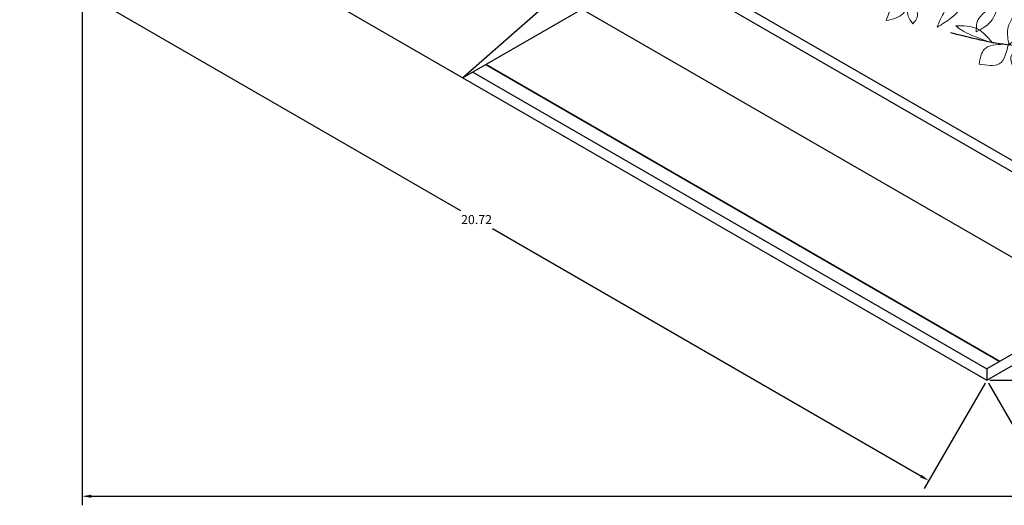
# Model space of a CAD drawing. Units: metres. Extents: x 12735 to 25554, y 20954 to 41989.
# Tile 1 of 15: x 12736.6 to 12756.13, y 20953.89 to 20963.53. Entities that reach past the tile are written whole.
import ezdxf

# ---------------------------------------------------------------- set-up
doc = ezdxf.new("R2010")
doc.units = ezdxf.units.M
doc.layers.get('Defpoints').update_dxf_attribs({"lineweight": 13})
for name, color, linetype, lineweight in [('A-ANNO-DIMS', 2, 'Continuous', 18), ('A-ELEV', 7, 'Continuous', 35), ('C-SITE', 8, 'Continuous', 25), ('TREES', 72, 'Continuous', 18)]:
    doc.layers.add(name, color=color, linetype=linetype, lineweight=lineweight)
doc.layers.add('STEM', color=32, linetype='Continuous')
doc.styles.get("Standard").update_dxf_attribs({"font": 'arial.ttf'})
doc.dimstyles.get("Standard").update_dxf_attribs({"dimtxt": 0.18, "dimasz": 0.18, "dimexe": 0.18, "dimexo": 0.0625, "dimgap": 0.09, "dimtad": 0, "dimtih": 1, "dimtoh": 1, "dimdec": 4, "dimzin": 0, "dimdsep": 46, "dimtxsty": 'Standard', "dimcen": 0.09, "dimadec": 0, "dimazin": 0, "dimtfac": 1, "dimtdec": 4, "dimtofl": 0, "dimtmove": 0, "dimatfit": 3, "dimfxl": 1, "dimtolj": 1, "dimtzin": 0, "dimarcsym": 0})

# ---------------------------------------------------------------- blocks, each defined once
blk = doc.blocks.new('TREES')
blk.add_line((12743.7, 20972.648), (12743.7, 20972.648))
at = {"layer": 'STEM'}
for points, knots in [([(12743.791, 20972.546), (12743.793, 20972.564), (12743.795, 20972.582), (12743.797, 20972.6), (12743.801, 20972.637), (12743.806, 20972.674), (12743.81, 20972.711), (12743.845, 20973.018), (12743.938, 20973.826), (12743.743, 20974.806), (12743.607, 20975.634), (12743.413, 20975.893), (12743.333, 20975.999)], [-0.164913, -0.164913, -0.164913, -0.164913, -0.110972, -0.110972, -0.110972, 0, 0, 0, 0.920963, 2.426088, 2.990404, 3.384799, 3.384799, 3.384799, 3.384799]), ([(12743.7, 20972.648), (12743.691, 20972.807), (12743.671, 20973.194), (12743.257, 20973.699), (12743.111, 20974.379), (12743.038, 20974.998), (12742.993, 20975.377), (12742.974, 20975.54)], [0, 0, 0, 0, 0.469346, 1.137622, 1.869488, 2.521439, 3.013071, 3.013071, 3.013071, 3.013071]), ([(12743.874, 20972.227), (12743.898, 20972.277), (12743.921, 20972.328), (12743.945, 20972.378), (12744.022, 20972.541), (12744.105, 20972.717), (12744.205, 20972.963), (12744.312, 20973.088), (12744.183, 20973.501), (12744.667, 20973.973), (12744.707, 20974.64), (12744.896, 20975.012), (12744.823, 20975.434), (12744.85, 20975.23), (12744.867, 20975.1)], [-0.166951, -0.166951, -0.166951, -0.166951, 0, 0, 0, 0.539768, 0.582066, 0.798222, 0.98781, 1.7696, 2.524754, 2.899414, 3.105113, 3.460848, 3.460848, 3.460848, 3.460848]), ([(12743.728, 20972.218), (12743.63, 20972.372), (12743.383, 20972.76), (12742.753, 20973.07), (12742.291, 20973.419), (12741.984, 20973.759), (12741.959, 20974.098), (12741.675, 20974.346), (12741.563, 20974.543), (12741.494, 20974.663)], [0, 0, 0, 0, 0.542161, 1.359078, 2.03444, 2.290187, 2.703676, 2.968549, 3.382864, 3.382864, 3.382864, 3.382864]), ([(12743.967, 20971.294), (12743.987, 20971.335), (12744.006, 20971.376), (12744.026, 20971.417), (12744.057, 20971.483), (12744.088, 20971.549), (12744.119, 20971.615), (12744.196, 20971.778), (12744.279, 20971.954), (12744.378, 20972.2), (12744.486, 20972.325), (12744.357, 20972.738), (12744.836, 20973.215), (12744.895, 20973.862), (12745.051, 20974.269), (12745.045, 20974.62), (12744.834, 20974.67), (12744.7, 20974.701)], [-0.355099, -0.355099, -0.355099, -0.355099, -0.218492, -0.218492, -0.218492, 0, 0, 0, 0.539768, 0.582066, 0.798222, 0.98781, 1.7696, 2.524754, 2.899414, 3.105113, 3.460848, 3.460848, 3.460848, 3.460848]), ([(12744.175, 20971.633), (12744.383, 20971.767), (12744.692, 20971.967), (12745.149, 20972.305), (12745.828, 20972.463), (12745.606, 20973.185), (12745.967, 20973.583), (12745.99, 20973.882), (12746.002, 20974.029)], [0, 0, 0, 0, 0.736164, 1.094646, 1.754618, 2.392389, 2.840214, 3.27091, 3.27091, 3.27091, 3.27091]), ([(12743.381, 20973.588), (12743.52, 20973.4), (12743.728, 20973.118), (12743.725, 20972.776), (12743.724, 20972.661), (12743.724, 20972.661), (12743.724, 20972.661), (12743.724, 20972.661), (12743.724, 20972.65), (12743.724, 20972.639), (12743.724, 20972.627)], [0, 0, 0, 0, 0.673099, 1.009429, 1.009429, 1.009429, 1.009429, 1.009429, 1.009429, 1.043412, 1.043412, 1.043412, 1.043412]), ([(12743.814, 20972.505), (12743.817, 20972.531), (12743.819, 20972.556), (12743.822, 20972.581), (12743.827, 20972.63), (12743.832, 20972.679), (12743.838, 20972.727), (12743.847, 20972.813), (12743.865, 20972.982), (12743.864, 20973.152), (12743.864, 20973.236)], [-0.2227932, -0.2227932, -0.2227932, -0.2227932, -0.1464713, -0.1464713, -0.1464713, 0, 0, 0, 0.2578951, 0.5103882, 0.5103882, 0.5103882, 0.5103882]), ([(12743.902, 20971.717), (12743.93, 20971.754), (12743.959, 20971.791), (12743.988, 20971.829), (12743.988, 20971.829), (12743.988, 20971.829), (12743.988, 20971.829), (12744.096, 20971.973), (12744.236, 20972.16), (12744.082, 20972.476), (12744.347, 20972.598), (12744.368, 20972.766), (12744.376, 20972.837)], [-0.129757, -0.129757, -0.129757, -0.129757, 0, 0, 0, 0, 0, 0, 0.485118, 0.62751, 0.913144, 1.120766, 1.120766, 1.120766, 1.120766]), ([(12744.111, 20968.725), (12743.967, 20969.837), (12743.799, 20971.142), (12743.712, 20972.453), (12743.7, 20972.648)], [0, 0, 0, 0, 3.359203, 3.944548, 3.944548, 3.944548, 3.944548]), ([(12744.332, 20968.825), (12744.189, 20969.936), (12743.871, 20971.161), (12743.872, 20972.51), (12743.7, 20972.648)], [0, 0, 0, 0, 3.359203, 3.972384, 3.972384, 3.972384, 3.972384]), ([(12743.597, 20972.418), (12743.533, 20972.41), (12743.292, 20972.379), (12742.889, 20972.351), (12742.364, 20972.241), (12741.803, 20972.489), (12741.157, 20972.302), (12740.698, 20972.258), (12740.474, 20972.237)], [0, 0, 0, 0, 0.193148, 0.727923, 1.218416, 1.762371, 2.471743, 3.152626, 3.152626, 3.152626, 3.152626]), ([(12743.181, 20972.372), (12743.296, 20972.37), (12743.441, 20972.368), (12743.583, 20972.39), (12743.613, 20972.395)], [0, 0, 0, 0, 0.3435042, 0.4329772, 0.4329772, 0.4329772, 0.4329772]), ([(12743.948, 20971.264), (12743.975, 20971.305), (12744.002, 20971.345), (12744.029, 20971.386), (12744.029, 20971.386), (12744.029, 20971.386), (12744.029, 20971.386), (12744.129, 20971.55), (12744.289, 20971.812), (12744.368, 20972.107), (12744.398, 20972.218)], [-0.148605, -0.148605, -0.148605, -0.148605, 0, 0, 0, 0, 0, 0, 0.572176, 0.914425, 0.914425, 0.914425, 0.914425]), ([(12743.901, 20971.729), (12743.929, 20971.768), (12743.958, 20971.808), (12743.986, 20971.847), (12743.986, 20971.847), (12743.986, 20971.847), (12743.986, 20971.847), (12744.02, 20971.892), (12744.062, 20971.951), (12744.099, 20972.014), (12744.107, 20972.028)], [-0.1467707, -0.1467707, -0.1467707, -0.1467707, 0, 0, 0, 0, 0, 0, 0.1684242, 0.2179474, 0.2179474, 0.2179474, 0.2179474]), ([(12743.81, 20971.258), (12743.646, 20971.316), (12743.283, 20971.443), (12742.486, 20971.453), (12741.888, 20971.61), (12741.494, 20971.714)], [0, 0, 0, 0, 0.519056, 1.146346, 2.366016, 2.366016, 2.366016, 2.366016])]:
    blk.add_open_spline(points, degree=3, knots=knots, dxfattribs=at)
blk.add_open_spline([(12744.644, 20971.941), (12744.672, 20971.961), (12744.701, 20971.98), (12744.73, 20972)], degree=3, dxfattribs=at)
at = {"layer": 'TREES'}
for points, knots in [([(12743.584, 20975.586), (12743.37, 20975.718), (12743.075, 20975.9), (12743.022, 20976.725), (12743.333, 20976.097), (12743.574, 20975.612)], [0, 0, 0, 0, 0.724771, 1.002271, 1.932196, 1.932196, 1.932196, 1.932196]), ([(12743.021, 20975.14), (12743.019, 20975.277), (12743.016, 20975.483), (12742.921, 20975.662), (12742.889, 20975.721)], [0, 0, 0, 0, 0.4023849, 0.6031293, 0.6031293, 0.6031293, 0.6031293]), ([(12743.021, 20975.14), (12742.985, 20975.224), (12742.928, 20975.356), (12742.766, 20975.539), (12742.854, 20975.638), (12742.901, 20975.69)], [0, 0, 0, 0, 0.2845416, 0.4465287, 0.6279758, 0.6279758, 0.6279758, 0.6279758]), ([(12743.718, 20974.979), (12743.671, 20975.164), (12743.598, 20975.454), (12743.323, 20975.534), (12743.223, 20975.563)], [0, 0, 0, 0, 0.519429, 0.8155501, 0.8155501, 0.8155501, 0.8155501]), ([(12743.223, 20975.563), (12743.266, 20975.448), (12743.36, 20975.195), (12743.592, 20975.055), (12743.718, 20974.979)], [0, 0, 0, 0, 0.3595778, 0.7860105, 0.7860105, 0.7860105, 0.7860105]), ([(12743.737, 20974.871), (12743.729, 20975.055), (12743.718, 20975.333), (12743.914, 20975.516), (12743.981, 20975.578)], [0, 0, 0, 0, 0.5134638, 0.7779111, 0.7779111, 0.7779111, 0.7779111]), ([(12743.737, 20974.871), (12743.801, 20974.971), (12743.939, 20975.186), (12743.966, 20975.441), (12743.981, 20975.578)], [0, 0, 0, 0, 0.351068, 0.7565079, 0.7565079, 0.7565079, 0.7565079]), ([(12741.648, 20974.411), (12741.519, 20974.547), (12741.281, 20974.798), (12741.642, 20974.995), (12741.673, 20975.511), (12741.684, 20975.149), (12741.787, 20975.033), (12741.768, 20974.824), (12741.781, 20974.575), (12741.641, 20974.411), (12741.569, 20974.326)], [0, 0, 0, 0, 0.446457, 0.821839, 1.096823, 1.294203, 1.491123, 1.594729, 1.894892, 2.216107, 2.216107, 2.216107, 2.216107]), ([(12743.07, 20974.733), (12742.98, 20974.863), (12742.848, 20975.053), (12742.433, 20975.446), (12742.649, 20974.915), (12742.651, 20974.573), (12742.961, 20974.576), (12743.034, 20974.678), (12743.071, 20974.73)], [0, 0, 0, 0, 0.54832, 0.799685, 1.166614, 1.565159, 1.742127, 1.925713, 1.925713, 1.925713, 1.925713]), ([(12743.031, 20975.058), (12743.048, 20975.139), (12743.077, 20975.281), (12743.184, 20975.377), (12743.231, 20975.418)], [0, 0, 0, 0, 0.2398723, 0.4207027, 0.4207027, 0.4207027, 0.4207027]), ([(12743.037, 20975.007), (12743.075, 20975.058), (12743.166, 20975.181), (12743.207, 20975.33), (12743.231, 20975.418)], [0, 0, 0, 0, 0.1895117, 0.457602, 0.457602, 0.457602, 0.457602]), ([(12744.796, 20974.806), (12744.757, 20974.909), (12744.688, 20975.088), (12744.514, 20975.28), (12744.523, 20975.414), (12744.526, 20975.464)], [0, 0, 0, 0, 0.3323117, 0.5782809, 0.7232611, 0.7232611, 0.7232611, 0.7232611]), ([(12744.805, 20974.813), (12744.804, 20974.918), (12744.803, 20975.076), (12744.822, 20975.37), (12744.643, 20975.427), (12744.526, 20975.464)], [0, 0, 0, 0, 0.3224266, 0.4885617, 0.8037384, 0.8037384, 0.8037384, 0.8037384]), ([(12744.796, 20974.806), (12744.882, 20974.878), (12745.017, 20974.992), (12745.211, 20975.15), (12745.228, 20975.277), (12745.236, 20975.337)], [0, 0, 0, 0, 0.3416822, 0.5370609, 0.7122352, 0.7122352, 0.7122352, 0.7122352]), ([(12744.839, 20974.951), (12744.859, 20975.055), (12744.903, 20975.272), (12745.122, 20975.315), (12745.236, 20975.337)], [0, 0, 0, 0, 0.2913456, 0.6064398, 0.6064398, 0.6064398, 0.6064398]), ([(12743.814, 20974.4), (12743.798, 20974.494), (12743.764, 20974.693), (12744.115, 20975.006), (12744.156, 20974.79), (12744.01, 20974.677), (12743.989, 20974.434), (12743.864, 20974.438), (12743.809, 20974.439)], [0, 0, 0, 0, 0.311146, 0.650746, 0.669061, 0.940573, 1.125337, 1.270427, 1.270427, 1.270427, 1.270427]), ([(12743.191, 20974.047), (12743.14, 20974.139), (12743.026, 20974.346), (12743.367, 20974.877), (12743.354, 20974.597), (12743.309, 20974.413), (12743.358, 20974.125), (12743.218, 20974.059), (12743.191, 20974.047)], [0, 0, 0, 0, 0.337622, 0.758697, 0.837919, 1.040495, 1.406258, 1.489574, 1.489574, 1.489574, 1.489574]), ([(12744.509, 20973.941), (12744.486, 20974.093), (12744.451, 20974.322), (12744.425, 20974.623), (12744.504, 20974.731), (12744.534, 20974.773)], [0, 0, 0, 0, 0.4681587, 0.7056034, 0.8580265, 0.8580265, 0.8580265, 0.8580265]), ([(12744.534, 20974.773), (12744.556, 20974.698), (12744.634, 20974.425), (12744.562, 20974.144), (12744.509, 20973.941)], [0, 0, 0, 0, 0.2327329, 0.8431329, 0.8431329, 0.8431329, 0.8431329]), ([(12744.554, 20973.975), (12744.669, 20974.016), (12744.893, 20974.094), (12745.019, 20974.421), (12745.06, 20974.624), (12745.08, 20974.72)], [0, 0, 0, 0, 0.348929, 0.678298, 0.9763146, 0.9763146, 0.9763146, 0.9763146]), ([(12742.028, 20973.754), (12742.003, 20973.912), (12741.953, 20974.218), (12742.174, 20974.414), (12742.283, 20974.81), (12742.258, 20974.48), (12742.304, 20974.323), (12742.246, 20974.069), (12742.227, 20973.932), (12742.006, 20973.671), (12742.066, 20973.72), (12742.075, 20973.727)], [0, 0, 0, 0, 0.436736, 0.842969, 1.012738, 1.21393, 1.403734, 1.613178, 1.897283, 2.067562, 2.097274, 2.097274, 2.097274, 2.097274]), ([(12743.835, 20974.249), (12743.789, 20974.346), (12743.724, 20974.484), (12743.556, 20974.594), (12743.468, 20974.601), (12743.424, 20974.604)], [0, 0, 0, 0, 0.3158223, 0.4463774, 0.5774617, 0.5774617, 0.5774617, 0.5774617]), ([(12743.424, 20974.604), (12743.442, 20974.527), (12743.487, 20974.324), (12743.715, 20974.191), (12743.841, 20974.206), (12743.841, 20974.206)], [0, 0, 0, 0, 0.2361186, 0.6165307, 0.6167763, 0.6167763, 0.6167763, 0.6167763]), ([(12744.618, 20974.118), (12744.717, 20974.268), (12744.844, 20974.462), (12745.022, 20974.606), (12745.062, 20974.638)], [0, 0, 0, 0, 0.5333846, 0.686651, 0.686651, 0.686651, 0.686651]), ([(12744.97, 20974.043), (12744.931, 20974.146), (12744.862, 20974.325), (12744.688, 20974.517), (12744.697, 20974.651), (12744.7, 20974.701)], [0, 0, 0, 0, 0.3323117, 0.5782809, 0.7232611, 0.7232611, 0.7232611, 0.7232611]), ([(12744.97, 20974.043), (12745.056, 20974.115), (12745.191, 20974.229), (12745.385, 20974.387), (12745.402, 20974.514), (12745.41, 20974.574)], [0, 0, 0, 0, 0.3416822, 0.5370609, 0.7122352, 0.7122352, 0.7122352, 0.7122352]), ([(12745.013, 20974.188), (12745.033, 20974.292), (12745.077, 20974.509), (12745.296, 20974.552), (12745.41, 20974.574)], [0, 0, 0, 0, 0.2913456, 0.6064398, 0.6064398, 0.6064398, 0.6064398]), ([(12745.957, 20973.706), (12745.908, 20973.835), (12745.798, 20974.123), (12745.864, 20974.427), (12745.9, 20974.594)], [0, 0, 0, 0, 0.4051126, 0.906838, 0.906838, 0.906838, 0.906838]), ([(12745.9, 20974.594), (12745.955, 20974.471), (12746.037, 20974.287), (12746.01, 20974.092), (12746.002, 20974.029)], [0, 0, 0, 0, 0.3943838, 0.5836156, 0.5836156, 0.5836156, 0.5836156]), ([(12743.128, 20974.182), (12743.019, 20974.275), (12742.841, 20974.427), (12742.65, 20974.313), (12742.577, 20974.27)], [0, 0, 0, 0, 0.3785086, 0.6144536, 0.6144536, 0.6144536, 0.6144536]), ([(12741.943, 20974.016), (12741.835, 20974.13), (12741.594, 20974.382), (12741.272, 20973.991), (12740.687, 20974.27), (12741.289, 20973.836), (12741.63, 20973.742), (12741.878, 20973.799), (12742.016, 20973.831)], [0, 0, 0, 0, 0.397812, 0.88569, 1.156328, 1.66735, 1.991498, 2.394837, 2.394837, 2.394837, 2.394837]), ([(12742.577, 20974.27), (12742.635, 20974.174), (12742.755, 20973.977), (12743.187, 20974.003), (12743.173, 20974.131), (12743.172, 20974.137)], [0, 0, 0, 0, 0.3386751, 0.6999446, 0.7185805, 0.7185805, 0.7185805, 0.7185805]), ([(12743.879, 20973.555), (12743.816, 20973.752), (12743.731, 20974.021), (12743.982, 20974.067), (12744.068, 20974.224), (12744.006, 20973.984), (12744.093, 20973.824), (12743.961, 20973.709), (12743.879, 20973.638)], [0, 0, 0, 0, 0.469961, 0.638827, 0.705595, 0.853148, 1.022788, 1.296962, 1.296962, 1.296962, 1.296962]), ([(12745.785, 20973.361), (12745.68, 20973.449), (12745.404, 20973.684), (12745.451, 20974.057), (12745.481, 20974.288)], [0, 0, 0, 0, 0.391493, 1.034106, 1.034106, 1.034106, 1.034106]), ([(12745.481, 20974.288), (12745.577, 20974.138), (12745.76, 20973.855), (12745.777, 20973.519), (12745.785, 20973.361)], [0, 0, 0, 0, 0.5245256, 0.9915723, 0.9915723, 0.9915723, 0.9915723]), ([(12742.389, 20973.356), (12742.341, 20973.437), (12742.234, 20973.617), (12742.458, 20973.799), (12742.48, 20973.946), (12742.486, 20973.991)], [0, 0, 0, 0, 0.251735, 0.5591808, 0.6938707, 0.6938707, 0.6938707, 0.6938707]), ([(12742.486, 20973.991), (12742.542, 20973.959), (12742.68, 20973.88), (12742.598, 20973.572), (12742.464, 20973.433), (12742.389, 20973.356)], [0, 0, 0, 0, 0.1746142, 0.4385715, 0.7703441, 0.7703441, 0.7703441, 0.7703441]), ([(12743.381, 20973.588), (12743.369, 20973.67), (12743.344, 20973.833), (12743.453, 20973.958), (12743.508, 20974.02)], [0, 0, 0, 0, 0.2360196, 0.4713289, 0.4713289, 0.4713289, 0.4713289]), ([(12743.381, 20973.588), (12743.434, 20973.649), (12743.541, 20973.774), (12743.519, 20973.937), (12743.508, 20974.02)], [0, 0, 0, 0, 0.2309694, 0.4699481, 0.4699481, 0.4699481, 0.4699481]), ([(12744.356, 20973.647), (12744.309, 20973.708), (12744.202, 20973.846), (12744.245, 20974.018), (12744.268, 20974.113)], [0, 0, 0, 0, 0.2209277, 0.4981889, 0.4981889, 0.4981889, 0.4981889]), ([(12744.268, 20974.113), (12744.323, 20974.065), (12744.46, 20973.94), (12744.395, 20973.758), (12744.356, 20973.647)], [0, 0, 0, 0, 0.203616, 0.5174389, 0.5174389, 0.5174389, 0.5174389]), ([(12744.683, 20973.178), (12744.66, 20973.33), (12744.625, 20973.559), (12744.599, 20973.86), (12744.677, 20973.968), (12744.708, 20974.01)], [0, 0, 0, 0, 0.4681587, 0.7056034, 0.8580265, 0.8580265, 0.8580265, 0.8580265]), ([(12744.708, 20974.01), (12744.73, 20973.935), (12744.807, 20973.662), (12744.735, 20973.381), (12744.683, 20973.178)], [0, 0, 0, 0, 0.2327329, 0.8431329, 0.8431329, 0.8431329, 0.8431329]), ([(12744.728, 20973.213), (12744.843, 20973.253), (12745.067, 20973.331), (12745.193, 20973.658), (12745.234, 20973.861), (12745.254, 20973.957)], [0, 0, 0, 0, 0.348929, 0.678298, 0.9763146, 0.9763146, 0.9763146, 0.9763146]), ([(12743.851, 20973.09), (12743.747, 20973.196), (12743.578, 20973.368), (12743.647, 20973.644), (12743.671, 20973.769), (12743.679, 20973.81)], [0, 0, 0, 0, 0.4076044, 0.6640272, 0.7921335, 0.7921335, 0.7921335, 0.7921335]), ([(12743.679, 20973.81), (12743.708, 20973.778), (12743.776, 20973.703), (12743.798, 20973.443), (12743.829, 20973.238), (12743.851, 20973.09)], [0, 0, 0, 0, 0.125659, 0.2981213, 0.7527794, 0.7527794, 0.7527794, 0.7527794]), ([(12744.792, 20973.355), (12744.891, 20973.505), (12745.018, 20973.699), (12745.196, 20973.843), (12745.236, 20973.876)], [0, 0, 0, 0, 0.5333846, 0.686651, 0.686651, 0.686651, 0.686651]), ([(12742.221, 20973.506), (12741.989, 20973.602), (12741.674, 20973.731), (12741.536, 20973.471), (12741.5, 20973.404)], [0, 0, 0, 0, 0.6060397, 0.8197481, 0.8197481, 0.8197481, 0.8197481]), ([(12743.253, 20972.784), (12743.147, 20972.854), (12742.919, 20973.005), (12742.8, 20973.728), (12742.973, 20973.491), (12743.022, 20973.422)], [0, 0, 0, 0, 0.420416, 0.90702, 1.103207, 1.103207, 1.103207, 1.103207]), ([(12743.364, 20973.617), (12743.288, 20973.661), (12743.124, 20973.754), (12742.939, 20973.715), (12742.84, 20973.694)], [0, 0, 0, 0, 0.2535199, 0.5460217, 0.5460217, 0.5460217, 0.5460217]), ([(12742.84, 20973.694), (12742.956, 20973.634), (12743.128, 20973.545), (12743.306, 20973.6), (12743.364, 20973.617)], [0, 0, 0, 0, 0.369417, 0.546183, 0.546183, 0.546183, 0.546183]), ([(12743.864, 20973.236), (12743.891, 20973.272), (12743.952, 20973.35), (12744.077, 20973.438), (12744.058, 20973.527), (12744.051, 20973.558)], [0, 0, 0, 0, 0.1377377, 0.3031534, 0.3935537, 0.3935537, 0.3935537, 0.3935537]), ([(12743.866, 20973.267), (12743.872, 20973.352), (12743.881, 20973.49), (12744.004, 20973.539), (12744.051, 20973.558)], [0, 0, 0, 0, 0.2295676, 0.3730638, 0.3730638, 0.3730638, 0.3730638]), ([(12744.268, 20973.425), (12744.32, 20973.505), (12744.424, 20973.666), (12744.615, 20973.662), (12744.711, 20973.66)], [0, 0, 0, 0, 0.2669279, 0.5349854, 0.5349854, 0.5349854, 0.5349854]), ([(12744.268, 20973.425), (12744.336, 20973.433), (12744.51, 20973.454), (12744.635, 20973.582), (12744.711, 20973.66)], [0, 0, 0, 0, 0.1990667, 0.5143408, 0.5143408, 0.5143408, 0.5143408]), ([(12741.493, 20973.429), (12741.634, 20973.396), (12741.906, 20973.333), (12742.16, 20973.449), (12742.283, 20973.505)], [0, 0, 0, 0, 0.420024, 0.8136231, 0.8136231, 0.8136231, 0.8136231]), ([(12743.022, 20973.422), (12743.059, 20973.426), (12743.334, 20973.456), (12743.256, 20972.956), (12743.349, 20972.723), (12743.36, 20972.696)], [0, 0, 0, 0, 0.1039343, 0.7792863, 0.8705393, 0.8705393, 0.8705393, 0.8705393]), ([(12744.53, 20972.884), (12744.482, 20972.945), (12744.376, 20973.084), (12744.419, 20973.255), (12744.442, 20973.351)], [0, 0, 0, 0, 0.2209277, 0.4981889, 0.4981889, 0.4981889, 0.4981889]), ([(12744.442, 20973.351), (12744.496, 20973.302), (12744.634, 20973.177), (12744.569, 20972.995), (12744.53, 20972.884)], [0, 0, 0, 0, 0.203616, 0.5174389, 0.5174389, 0.5174389, 0.5174389]), ([(12745.697, 20972.996), (12745.547, 20972.999), (12745.238, 20973.004), (12745.268, 20973.314), (12745.283, 20973.473)], [0, 0, 0, 0, 0.3799868, 0.779071, 0.779071, 0.779071, 0.779071]), ([(12745.283, 20973.473), (12745.354, 20973.458), (12745.585, 20973.409), (12745.651, 20973.165), (12745.697, 20972.996)], [0, 0, 0, 0, 0.2074949, 0.6743984, 0.6743984, 0.6743984, 0.6743984]), ([(12741.595, 20972.406), (12741.523, 20972.496), (12741.318, 20972.752), (12741.336, 20973.087), (12741.348, 20973.304)], [0, 0, 0, 0, 0.3390919, 0.9589007, 0.9589007, 0.9589007, 0.9589007]), ([(12741.348, 20973.304), (12741.406, 20973.227), (12741.6, 20972.969), (12741.591, 20972.637), (12741.585, 20972.405)], [0, 0, 0, 0, 0.2865181, 0.9509807, 0.9509807, 0.9509807, 0.9509807]), ([(12743.621, 20973.151), (12743.561, 20973.233), (12743.473, 20973.354), (12743.333, 20973.334), (12743.288, 20973.327)], [0, 0, 0, 0, 0.2726158, 0.4022356, 0.4022356, 0.4022356, 0.4022356]), ([(12743.288, 20973.327), (12743.325, 20973.265), (12743.399, 20973.138), (12743.546, 20973.147), (12743.621, 20973.151)], [0, 0, 0, 0, 0.199886, 0.4070645, 0.4070645, 0.4070645, 0.4070645]), ([(12744.074, 20972.655), (12744.086, 20972.673), (12744.124, 20972.731), (12743.998, 20972.782), (12744.014, 20972.867), (12744.011, 20972.925), (12744.052, 20972.944), (12744.07, 20973.015), (12743.988, 20973.027), (12743.97, 20973.091), (12744.03, 20973.11), (12744.072, 20973.132), (12744.097, 20973.169), (12744.133, 20973.163), (12744.172, 20973.164), (12744.216, 20973.136), (12744.296, 20973.17), (12744.282, 20973.105), (12744.259, 20973.057), (12744.341, 20973.048), (12744.328, 20972.986), (12744.32, 20972.935), (12744.299, 20972.884), (12744.258, 20972.852), (12744.236, 20972.821), (12744.215, 20972.805), (12744.179, 20972.793), (12744.139, 20972.807), (12744.095, 20972.746), (12744.111, 20972.739), (12744.111, 20972.739)], [0, 0, 0, 0, 0.055886, 0.185472, 0.25227, 0.305988, 0.338368, 0.378405, 0.48523, 0.4997, 0.565031, 0.618654, 0.656012, 0.680602, 0.71942, 0.77395, 0.836088, 0.890088, 0.913694, 0.979696, 1.032481, 1.0683, 1.142133, 1.186825, 1.224162, 1.25438, 1.26551, 1.333296, 1.383591, 1.385324, 1.385324, 1.385324, 1.385324]), ([(12745.697, 20972.996), (12745.724, 20973.08), (12745.77, 20973.226), (12745.915, 20973.262), (12745.976, 20973.277)], [0, 0, 0, 0, 0.2439478, 0.4222058, 0.4222058, 0.4222058, 0.4222058]), ([(12745.697, 20972.996), (12745.764, 20973.024), (12745.897, 20973.078), (12745.95, 20973.211), (12745.976, 20973.277)], [0, 0, 0, 0, 0.2073861, 0.4117039, 0.4117039, 0.4117039, 0.4117039]), ([(12742.983, 20972.961), (12742.799, 20973.009), (12742.463, 20973.098), (12742.071, 20972.928), (12741.893, 20972.798), (12741.839, 20972.759)], [0, 0, 0, 0, 0.553894, 1.01265, 1.215779, 1.215779, 1.215779, 1.215779]), ([(12741.839, 20972.759), (12741.949, 20972.7), (12742.323, 20972.501), (12742.684, 20972.786), (12742.939, 20972.987)], [0, 0, 0, 0, 0.355589, 1.206871, 1.206871, 1.206871, 1.206871]), ([(12743.669, 20972.977), (12743.606, 20973.025), (12743.504, 20973.102), (12743.398, 20973.043), (12743.358, 20973.021)], [0, 0, 0, 0, 0.2119595, 0.340544, 0.340544, 0.340544, 0.340544]), ([(12743.358, 20973.021), (12743.426, 20972.983), (12743.527, 20972.926), (12743.633, 20972.964), (12743.669, 20972.977)], [0, 0, 0, 0, 0.2166399, 0.3265492, 0.3265492, 0.3265492, 0.3265492]), ([(12741.358, 20972.366), (12741.291, 20972.434), (12741.162, 20972.564), (12740.909, 20972.646), (12740.492, 20972.989), (12740.719, 20972.381), (12740.905, 20972.253), (12741.437, 20972.382), (12741.361, 20972.366), (12741.358, 20972.366)], [0, 0, 0, 0, 0.274554, 0.529523, 0.902439, 1.220606, 1.740632, 1.953969, 1.962894, 1.962894, 1.962894, 1.962894]), ([(12743.257, 20972.379), (12743.071, 20972.409), (12742.794, 20972.453), (12742.842, 20972.698), (12742.858, 20972.779)], [0, 0, 0, 0, 0.4478858, 0.6692237, 0.6692237, 0.6692237, 0.6692237]), ([(12742.858, 20972.779), (12743.034, 20972.81), (12743.375, 20972.87), (12743.295, 20972.539), (12743.257, 20972.379)], [0, 0, 0, 0, 0.4156133, 0.8046117, 0.8046117, 0.8046117, 0.8046117]), ([(12744.299, 20972.615), (12744.284, 20972.657), (12744.255, 20972.734), (12744.322, 20972.816), (12744.34, 20972.869), (12744.347, 20972.89)], [0, 0, 0, 0, 0.1248577, 0.2264879, 0.2926557, 0.2926557, 0.2926557, 0.2926557]), ([(12744.442, 20972.662), (12744.494, 20972.743), (12744.598, 20972.903), (12744.789, 20972.899), (12744.885, 20972.897)], [0, 0, 0, 0, 0.2669279, 0.5349854, 0.5349854, 0.5349854, 0.5349854]), ([(12744.442, 20972.662), (12744.51, 20972.671), (12744.684, 20972.691), (12744.809, 20972.819), (12744.885, 20972.897)], [0, 0, 0, 0, 0.1990667, 0.5143408, 0.5143408, 0.5143408, 0.5143408]), ([(12745.557, 20972.46), (12745.505, 20972.545), (12745.415, 20972.69), (12745.509, 20972.826), (12745.548, 20972.882)], [0, 0, 0, 0, 0.2672291, 0.4594629, 0.4594629, 0.4594629, 0.4594629]), ([(12745.548, 20972.882), (12745.623, 20972.785), (12745.735, 20972.639), (12745.619, 20972.519), (12745.581, 20972.479)], [0, 0, 0, 0, 0.3063433, 0.4579535, 0.4579535, 0.4579535, 0.4579535]), ([(12745.681, 20972.634), (12745.776, 20972.643), (12745.97, 20972.661), (12746.056, 20972.838), (12746.1, 20972.929)], [0, 0, 0, 0, 0.2646598, 0.5464061, 0.5464061, 0.5464061, 0.5464061]), ([(12745.691, 20972.679), (12745.723, 20972.743), (12745.803, 20972.904), (12745.989, 20972.919), (12746.1, 20972.929)], [0, 0, 0, 0, 0.2025395, 0.5100625, 0.5100625, 0.5100625, 0.5100625]), ([(12740.645, 20972.254), (12740.532, 20972.287), (12740.33, 20972.345), (12740.37, 20972.543), (12740.387, 20972.63)], [0, 0, 0, 0, 0.300298, 0.5327787, 0.5327787, 0.5327787, 0.5327787]), ([(12740.387, 20972.63), (12740.446, 20972.602), (12740.598, 20972.53), (12740.627, 20972.359), (12740.645, 20972.254)], [0, 0, 0, 0, 0.1847401, 0.4807235, 0.4807235, 0.4807235, 0.4807235]), ([(12742.916, 20972.343), (12742.772, 20972.452), (12742.448, 20972.697), (12742.076, 20972.511), (12741.869, 20972.407)], [0, 0, 0, 0, 0.501704, 1.133573, 1.133573, 1.133573, 1.133573]), ([(12744.14, 20972.455), (12744.129, 20972.498), (12744.112, 20972.571), (12744.173, 20972.643), (12744.195, 20972.684), (12744.204, 20972.7)], [0, 0, 0, 0, 0.124617, 0.2107396, 0.2658134, 0.2658134, 0.2658134, 0.2658134]), ([(12744.14, 20972.455), (12744.155, 20972.485), (12744.181, 20972.535), (12744.225, 20972.615), (12744.212, 20972.669), (12744.204, 20972.7)], [0, 0, 0, 0, 0.1037237, 0.1704768, 0.2630686, 0.2630686, 0.2630686, 0.2630686]), ([(12744.192, 20972.515), (12744.244, 20972.502), (12744.335, 20972.479), (12744.372, 20972.56), (12744.387, 20972.593)], [0, 0, 0, 0, 0.1401829, 0.239855, 0.239855, 0.239855, 0.239855]), ([(12744.25, 20972.55), (12744.272, 20972.566), (12744.314, 20972.595), (12744.364, 20972.594), (12744.387, 20972.593)], [0, 0, 0, 0, 0.0790636, 0.1468534, 0.1468534, 0.1468534, 0.1468534]), ([(12745.276, 20972.317), (12745.252, 20972.391), (12745.204, 20972.544), (12745.32, 20972.655), (12745.379, 20972.712)], [0, 0, 0, 0, 0.2148949, 0.4418034, 0.4418034, 0.4418034, 0.4418034]), ([(12745.276, 20972.317), (12745.329, 20972.378), (12745.429, 20972.493), (12745.395, 20972.642), (12745.379, 20972.712)], [0, 0, 0, 0, 0.2259484, 0.4304915, 0.4304915, 0.4304915, 0.4304915]), ([(12741.223, 20971.823), (12741.319, 20971.881), (12741.571, 20972.033), (12741.755, 20972.264), (12741.869, 20972.407)], [0, 0, 0, 0, 0.3340001, 0.876507, 0.876507, 0.876507, 0.876507]), ([(12741.595, 20972.406), (12741.515, 20972.319), (12741.356, 20972.147), (12741.267, 20971.93), (12741.223, 20971.823)], [0, 0, 0, 0, 0.3521388, 0.6963584, 0.6963584, 0.6963584, 0.6963584]), ([(12744.145, 20972.348), (12744.132, 20972.384), (12744.105, 20972.455), (12744.032, 20972.434), (12743.996, 20972.423)], [0, 0, 0, 0, 0.098996, 0.196743, 0.196743, 0.196743, 0.196743]), ([(12743.996, 20972.423), (12744.027, 20972.377), (12744.069, 20972.315), (12744.13, 20972.341), (12744.146, 20972.347)], [0, 0, 0, 0, 0.1368513, 0.185287, 0.185287, 0.185287, 0.185287]), ([(12744.137, 20972.378), (12744.147, 20972.414), (12744.168, 20972.49), (12744.249, 20972.485), (12744.292, 20972.483)], [0, 0, 0, 0, 0.0982704, 0.2114853, 0.2114853, 0.2114853, 0.2114853]), ([(12744.137, 20972.378), (12744.171, 20972.382), (12744.241, 20972.388), (12744.274, 20972.45), (12744.292, 20972.483)], [0, 0, 0, 0, 0.0955829, 0.1975677, 0.1975677, 0.1975677, 0.1975677]), ([(12744.868, 20972.097), (12744.937, 20972.148), (12745.072, 20972.246), (12745.072, 20972.413), (12745.073, 20972.494)], [0, 0, 0, 0, 0.2403434, 0.4714363, 0.4714363, 0.4714363, 0.4714363]), ([(12744.868, 20972.097), (12744.895, 20972.212), (12744.931, 20972.363), (12745.046, 20972.458), (12745.074, 20972.481)], [0, 0, 0, 0, 0.3374321, 0.4432568, 0.4432568, 0.4432568, 0.4432568]), ([(12745.422, 20972.381), (12745.493, 20972.379), (12745.657, 20972.373), (12745.791, 20972.276), (12745.866, 20972.222)], [0, 0, 0, 0, 0.2087211, 0.4811791, 0.4811791, 0.4811791, 0.4811791]), ([(12745.422, 20972.381), (12745.521, 20972.247), (12745.661, 20972.058), (12745.82, 20972.185), (12745.866, 20972.222)], [0, 0, 0, 0, 0.3912381, 0.5526272, 0.5526272, 0.5526272, 0.5526272]), ([(12745.582, 20972.481), (12745.667, 20972.516), (12745.814, 20972.576), (12745.958, 20972.516), (12746.019, 20972.491)], [0, 0, 0, 0, 0.2625898, 0.453199, 0.453199, 0.453199, 0.453199]), ([(12745.582, 20972.481), (12745.658, 20972.433), (12745.808, 20972.341), (12745.95, 20972.442), (12746.019, 20972.491)], [0, 0, 0, 0, 0.2451587, 0.4783488, 0.4783488, 0.4783488, 0.4783488]), ([(12740.645, 20972.254), (12740.54, 20972.264), (12740.318, 20972.286), (12740.252, 20972.07), (12740.216, 20971.955)], [0, 0, 0, 0, 0.2808571, 0.5946199, 0.5946199, 0.5946199, 0.5946199]), ([(12740.216, 20971.955), (12740.344, 20971.984), (12740.536, 20972.026), (12740.618, 20972.197), (12740.645, 20972.254)], [0, 0, 0, 0, 0.3624795, 0.5464116, 0.5464116, 0.5464116, 0.5464116]), ([(12740.757, 20972.265), (12740.712, 20972.237), (12740.573, 20972.15), (12740.673, 20971.993), (12740.741, 20971.887)], [0, 0, 0, 0, 0.1417373, 0.4445248, 0.4445248, 0.4445248, 0.4445248]), ([(12740.741, 20971.887), (12740.783, 20971.937), (12740.878, 20972.054), (12740.801, 20972.189), (12740.757, 20972.265)], [0, 0, 0, 0, 0.1798963, 0.4162104, 0.4162104, 0.4162104, 0.4162104]), ([(12742.453, 20972.29), (12742.257, 20972.189), (12741.999, 20972.056), (12742.001, 20971.792), (12742.002, 20971.729)], [0, 0, 0, 0, 0.5792647, 0.7616052, 0.7616052, 0.7616052, 0.7616052]), ([(12742.002, 20971.729), (12742.108, 20971.788), (12742.333, 20971.914), (12742.411, 20972.161), (12742.453, 20972.29)], [0, 0, 0, 0, 0.3533474, 0.7448355, 0.7448355, 0.7448355, 0.7448355]), ([(12743.181, 20972.372), (12743.094, 20972.305), (12742.907, 20972.162), (12742.991, 20971.938), (12743.035, 20971.819)], [0, 0, 0, 0, 0.2977969, 0.6372286, 0.6372286, 0.6372286, 0.6372286]), ([(12743.035, 20971.819), (12743.147, 20971.88), (12743.383, 20972.009), (12743.25, 20972.247), (12743.181, 20972.372)], [0, 0, 0, 0, 0.3275492, 0.688496, 0.688496, 0.688496, 0.688496]), ([(12744.116, 20972.018), (12744.075, 20972.065), (12744.007, 20972.143), (12744.05, 20972.231), (12744.028, 20972.351), (12744.072, 20972.271), (12744.09, 20972.201), (12744.221, 20972.106), (12744.146, 20972.042), (12744.116, 20972.018)], [0, 0, 0, 0, 0.1633748, 0.2727914, 0.3326965, 0.376171, 0.4524353, 0.6040881, 0.701786, 0.701786, 0.701786, 0.701786]), ([(12744.455, 20971.815), (12744.445, 20971.868), (12744.427, 20971.97), (12744.523, 20972.088), (12744.564, 20972.169), (12744.585, 20972.208)], [0, 0, 0, 0, 0.1538132, 0.2966411, 0.4292928, 0.4292928, 0.4292928, 0.4292928]), ([(12744.455, 20971.815), (12744.544, 20971.891), (12744.679, 20972.008), (12744.609, 20972.157), (12744.585, 20972.208)], [0, 0, 0, 0, 0.3019229, 0.4589929, 0.4589929, 0.4589929, 0.4589929]), ([(12744.746, 20972.012), (12744.742, 20972.047), (12744.733, 20972.118), (12744.771, 20972.218), (12744.826, 20972.252), (12744.849, 20972.268)], [0, 0, 0, 0, 0.1066556, 0.2131282, 0.2966333, 0.2966333, 0.2966333, 0.2966333]), ([(12744.746, 20972.012), (12744.773, 20972.045), (12744.822, 20972.105), (12744.891, 20972.268), (12744.848, 20972.268), (12744.847, 20972.268)], [0, 0, 0, 0, 0.1585708, 0.2833525, 0.285588, 0.285588, 0.285588, 0.285588]), ([(12745.053, 20972.215), (12745.111, 20972.233), (12745.273, 20972.284), (12745.353, 20972.117), (12745.405, 20972.009)], [0, 0, 0, 0, 0.1646898, 0.4645687, 0.4645687, 0.4645687, 0.4645687]), ([(12745.053, 20972.215), (12745.087, 20972.171), (12745.174, 20972.057), (12745.317, 20972.027), (12745.405, 20972.009)], [0, 0, 0, 0, 0.1638697, 0.4194041, 0.4194041, 0.4194041, 0.4194041]), ([(12742.652, 20971.471), (12742.63, 20971.58), (12742.585, 20971.809), (12742.714, 20972.005), (12742.781, 20972.107)], [0, 0, 0, 0, 0.3207709, 0.6721329, 0.6721329, 0.6721329, 0.6721329]), ([(12742.652, 20971.471), (12742.732, 20971.545), (12742.92, 20971.718), (12742.832, 20971.965), (12742.781, 20972.107)], [0, 0, 0, 0, 0.3028446, 0.7080533, 0.7080533, 0.7080533, 0.7080533]), ([(12742.314, 20971.521), (12742.225, 20971.627), (12742.039, 20971.851), (12741.746, 20971.851), (12741.593, 20971.851)], [0, 0, 0, 0, 0.3968877, 0.8302181, 0.8302181, 0.8302181, 0.8302181]), ([(12741.593, 20971.851), (12741.666, 20971.793), (12741.821, 20971.668), (12742.447, 20971.471), (12742.312, 20971.521), (12742.311, 20971.521)], [0, 0, 0, 0, 0.3696351, 0.7965164, 0.7990281, 0.7990281, 0.7990281, 0.7990281]), ([(12743.566, 20971.341), (12743.514, 20971.414), (12743.424, 20971.54), (12743.418, 20971.749), (12743.449, 20971.857), (12743.463, 20971.904)], [0, 0, 0, 0, 0.2632417, 0.4527737, 0.6011812, 0.6011812, 0.6011812, 0.6011812]), ([(12743.463, 20971.904), (12743.567, 20971.861), (12743.772, 20971.775), (12743.623, 20971.516), (12743.587, 20971.385), (12743.574, 20971.338)], [0, 0, 0, 0, 0.2799093, 0.5517077, 0.7021324, 0.7021324, 0.7021324, 0.7021324]), ([(12744.561, 20971.885), (12744.589, 20971.902), (12744.651, 20971.938), (12744.742, 20971.883), (12744.801, 20971.859), (12744.827, 20971.849)], [0, 0, 0, 0, 0.0920276, 0.2010844, 0.2860976, 0.2860976, 0.2860976, 0.2860976]), ([(12744.561, 20971.885), (12744.599, 20971.871), (12744.674, 20971.844), (12744.795, 20971.792), (12744.822, 20971.84), (12744.827, 20971.849)], [0, 0, 0, 0, 0.1330667, 0.2587888, 0.2884885, 0.2884885, 0.2884885, 0.2884885]), ([(12743.304, 20971.408), (12743.247, 20971.446), (12743.157, 20971.505), (12743.12, 20971.647), (12743.123, 20971.722), (12743.125, 20971.759)], [0, 0, 0, 0, 0.196607, 0.3084716, 0.4203856, 0.4203856, 0.4203856, 0.4203856]), ([(12743.125, 20971.759), (12743.154, 20971.73), (12743.251, 20971.635), (12743.282, 20971.501), (12743.304, 20971.408)], [0, 0, 0, 0, 0.1222515, 0.400195, 0.400195, 0.400195, 0.400195]), ([(12742.056, 20971.092), (12742.207, 20971.066), (12742.53, 20971.009), (12742.604, 20971.335), (12742.644, 20971.51)], [0, 0, 0, 0, 0.3982442, 0.8534889, 0.8534889, 0.8534889, 0.8534889]), ([(12742.547, 20971.484), (12742.396, 20971.478), (12742.124, 20971.467), (12742.077, 20971.207), (12742.056, 20971.092)], [0, 0, 0, 0, 0.3960722, 0.7115037, 0.7115037, 0.7115037, 0.7115037]), ([(12742.918, 20971.429), (12742.811, 20971.373), (12742.636, 20971.282), (12742.7, 20971.111), (12742.725, 20971.045)], [0, 0, 0, 0, 0.3055467, 0.4944991, 0.4944991, 0.4944991, 0.4944991]), ([(12742.725, 20971.045), (12742.787, 20971.086), (12742.922, 20971.175), (12742.92, 20971.34), (12742.918, 20971.429)], [0, 0, 0, 0, 0.2088213, 0.4571427, 0.4571427, 0.4571427, 0.4571427]), ([(12743.381, 20971.391), (12743.311, 20971.354), (12743.137, 20971.26), (12743.15, 20971.056), (12743.158, 20970.935)], [0, 0, 0, 0, 0.2232821, 0.551466, 0.551466, 0.551466, 0.551466]), ([(12743.158, 20970.935), (12743.238, 20970.974), (12743.421, 20971.065), (12743.396, 20971.274), (12743.381, 20971.391)], [0, 0, 0, 0, 0.2445355, 0.5611675, 0.5611675, 0.5611675, 0.5611675]), ([(12743.743, 20971.282), (12743.611, 20971.245), (12743.396, 20971.185), (12743.421, 20970.978), (12743.431, 20970.898)], [0, 0, 0, 0, 0.3473993, 0.565418, 0.565418, 0.565418, 0.565418]), ([(12743.431, 20970.898), (12743.517, 20970.939), (12743.683, 20971.018), (12743.723, 20971.196), (12743.743, 20971.282)], [0, 0, 0, 0, 0.2699816, 0.5191769, 0.5191769, 0.5191769, 0.5191769])]:
    blk.add_open_spline(points, degree=3, knots=knots, dxfattribs=at)
blk.add_open_spline([(12744.347, 20972.89), (12744.357, 20972.872), (12744.367, 20972.854), (12744.376, 20972.837)], degree=3, dxfattribs=at)
blk = doc.blocks.new('*D9')
at = {"layer": 'A-ANNO-DIMS', "color": 0, "lineweight": -2, "transparency": 16777216}
for p, q in [((12781.004, 20970.87), (12781.004, 20953.893)), ((12737.843, 20966.671), (12737.843, 20953.893)), ((12738.023, 20954.073), (12759.026, 20954.073)), ((12780.824, 20954.073), (12759.821, 20954.073))]:
    blk.add_line(p, q, dxfattribs=at)
at = {"layer": 'A-ANNO-DIMS', "color": 0, "transparency": 16777216}
for points in [[(12738.023, 20954.103), (12738.023, 20954.043), (12737.843, 20954.073)], [(12780.824, 20954.103), (12780.824, 20954.043), (12781.004, 20954.073)]]:
    blk.add_solid(points, dxfattribs=at)
at = {"layer": 'Defpoints', "color": 0, "transparency": 16777216}
for p in [(12781.004, 20970.933), (12737.843, 20966.733), (12781.004, 20954.073)]:
    blk.add_point(p, dxfattribs=at)
at = {"layer": 'A-ANNO-DIMS', "color": 0, "transparency": 16777216, "insert": (12759.423, 20954.073), "char_height": 0.18, "attachment_point": 5}
blk.add_mtext('\\A1;43.16', dxfattribs=at)
blk = doc.blocks.new('*D10')
at = {"layer": 'A-ANNO-DIMS', "color": 0, "lineweight": -2, "transparency": 16777216}
for p, q in [((12766.645, 20994.825), (12783.484, 20994.825)), ((12783.304, 20994.645), (12783.304, 20975.781)), ((12783.304, 20956.553), (12783.304, 20975.417)), ((12755.849, 20956.373), (12783.484, 20956.373))]:
    blk.add_line(p, q, dxfattribs=at)
at = {"layer": 'A-ANNO-DIMS', "color": 0, "transparency": 16777216}
for points in [[(12783.274, 20994.645), (12783.334, 20994.645), (12783.304, 20994.825)], [(12783.274, 20956.553), (12783.334, 20956.553), (12783.304, 20956.373)]]:
    blk.add_solid(points, dxfattribs=at)
at = {"layer": 'Defpoints', "color": 0, "transparency": 16777216}
for p in [(12766.582, 20994.825), (12783.304, 20994.825), (12755.787, 20956.373)]:
    blk.add_point(p, dxfattribs=at)
at = {"layer": 'A-ANNO-DIMS', "color": 0, "transparency": 16777216, "insert": (12783.304, 20975.599), "char_height": 0.18, "attachment_point": 5}
blk.add_mtext('\\A1;38.45', dxfattribs=at)
blk = doc.blocks.new('*D11')
at = {"layer": 'A-ANNO-DIMS', "color": 0, "lineweight": -2, "transparency": 16777216}
for p, q in [((12737.811, 20966.679), (12736.603, 20964.586)), ((12736.848, 20964.652), (12745.35, 20959.743)), ((12754.481, 20954.472), (12745.98, 20959.38)), ((12755.756, 20956.319), (12754.547, 20954.226))]:
    blk.add_line(p, q, dxfattribs=at)
at = {"layer": 'A-ANNO-DIMS', "color": 0, "transparency": 16777216}
for points in [[(12736.863, 20964.678), (12736.833, 20964.626), (12736.693, 20964.742)], [(12754.496, 20954.497), (12754.466, 20954.446), (12754.637, 20954.382)]]:
    blk.add_solid(points, dxfattribs=at)
at = {"layer": 'Defpoints', "color": 0, "transparency": 16777216}
for p in [(12737.843, 20966.733), (12736.693, 20964.742), (12755.787, 20956.373)]:
    blk.add_point(p, dxfattribs=at)
at = {"layer": 'A-ANNO-DIMS', "color": 0, "transparency": 16777216, "insert": (12745.665, 20959.562), "char_height": 0.18, "attachment_point": 5}
blk.add_mtext('\\A1;20.72', dxfattribs=at)
blk = doc.blocks.new('*D12')
at = {"layer": 'A-ANNO-DIMS', "color": 0, "lineweight": -2, "transparency": 16777216}
for p, q in [((12781.035, 20970.878), (12782.244, 20968.785)), ((12781.998, 20968.851), (12769.861, 20961.843)), ((12757.093, 20954.472), (12769.23, 20961.479)), ((12755.818, 20956.319), (12757.027, 20954.226))]:
    blk.add_line(p, q, dxfattribs=at)
at = {"layer": 'A-ANNO-DIMS', "color": 0, "transparency": 16777216}
for points in [[(12781.983, 20968.877), (12782.013, 20968.825), (12782.154, 20968.941)], [(12757.078, 20954.497), (12757.108, 20954.446), (12756.937, 20954.382)]]:
    blk.add_solid(points, dxfattribs=at)
at = {"layer": 'Defpoints', "color": 0, "transparency": 16777216}
for p in [(12781.004, 20970.933), (12755.787, 20956.373), (12756.937, 20954.382)]:
    blk.add_point(p, dxfattribs=at)
at = {"layer": 'A-ANNO-DIMS', "color": 0, "transparency": 16777216, "insert": (12769.545, 20961.661), "char_height": 0.18, "attachment_point": 5}
blk.add_mtext('\\A1;29.12', dxfattribs=at)

msp = doc.modelspace()

# ---------------------------------------------------------------- linework, layer by layer
at = {"layer": 'A-ELEV'}
msp.add_line((12745.852, 20962.6352), (12756.0467, 20956.7494), dxfattribs=at)
at = {"layer": 'C-SITE'}
for p, q in [((12781.0041, 20971.1586), (12755.7869, 20956.5994)), ((12755.7869, 20956.3734), (12781.0041, 20970.9326)), ((12757.9519, 20957.8494), (12740.0077, 20968.2095)), ((12737.8426, 20966.7335), (12755.7869, 20956.3734)), ((12747.953, 20965.5482), (12757.9519, 20959.7754)), ((12747.7573, 20965.4352), (12757.9519, 20959.5494)), ((12747.4196, 20964.1562), (12745.3965, 20962.3722)), ((12747.7573, 20963.7352), (12745.3965, 20962.3722)), ((12745.5922, 20962.4852), (12755.7869, 20956.5994)), ((12755.7869, 20956.5994), (12755.7869, 20956.3734))]:
    msp.add_line(p, q, dxfattribs=at)

# ---------------------------------------------------------------- block references
at = {"layer": 'TREES'}
msp.add_blockref('TREES', (13.5777, -8.4449), dxfattribs=at)

# ---------------------------------------------------------------- dimensions: what is measured, and where the dimension line sits
at = {"layer": 'A-ANNO-DIMS'}
for base, p1, p2, angle, picture, middle in [((12783.3041, 20994.8247), (12755.7869, 20956.3734), (12766.582, 20994.8247), 90, '*D10', (12783.3041, 20975.599)), ((12756.9369, 20954.3815), (12781.0041, 20970.9326), (12755.7869, 20956.3734), 210, '*D12', (12769.5455, 20961.6611)), ((12736.6926, 20964.7416), (12755.7869, 20956.3734), (12737.8426, 20966.7335), 150, '*D11', (12745.6647, 20959.5616))]:
    dim = msp.add_linear_dim(base=base, p1=p1, p2=p2, angle=angle, dimstyle='Standard', override={"dimdec": 2, "dimlfac": 1, "dimrnd": 0, "dimzin": 0, "dimdsep": 46, "dimlunit": 2}, dxfattribs=at)
    dim.commit()
    dim.dimension.update_dxf_attribs({"geometry": picture, "text_midpoint": middle})
dim = msp.add_linear_dim(base=(12781.0041, 20954.0734), p1=(12737.8426, 20966.7335), p2=(12781.0041, 20970.9326), dimstyle='Standard', override={"dimdec": 2, "dimlfac": 1, "dimrnd": 0, "dimzin": 0, "dimdsep": 46, "dimlunit": 2}, dxfattribs=at)
dim.commit()
dim.dimension.update_dxf_attribs({"geometry": '*D9', "text_midpoint": (12759.4234, 20954.0734)})

doc.saveas('drawing.dxf')
